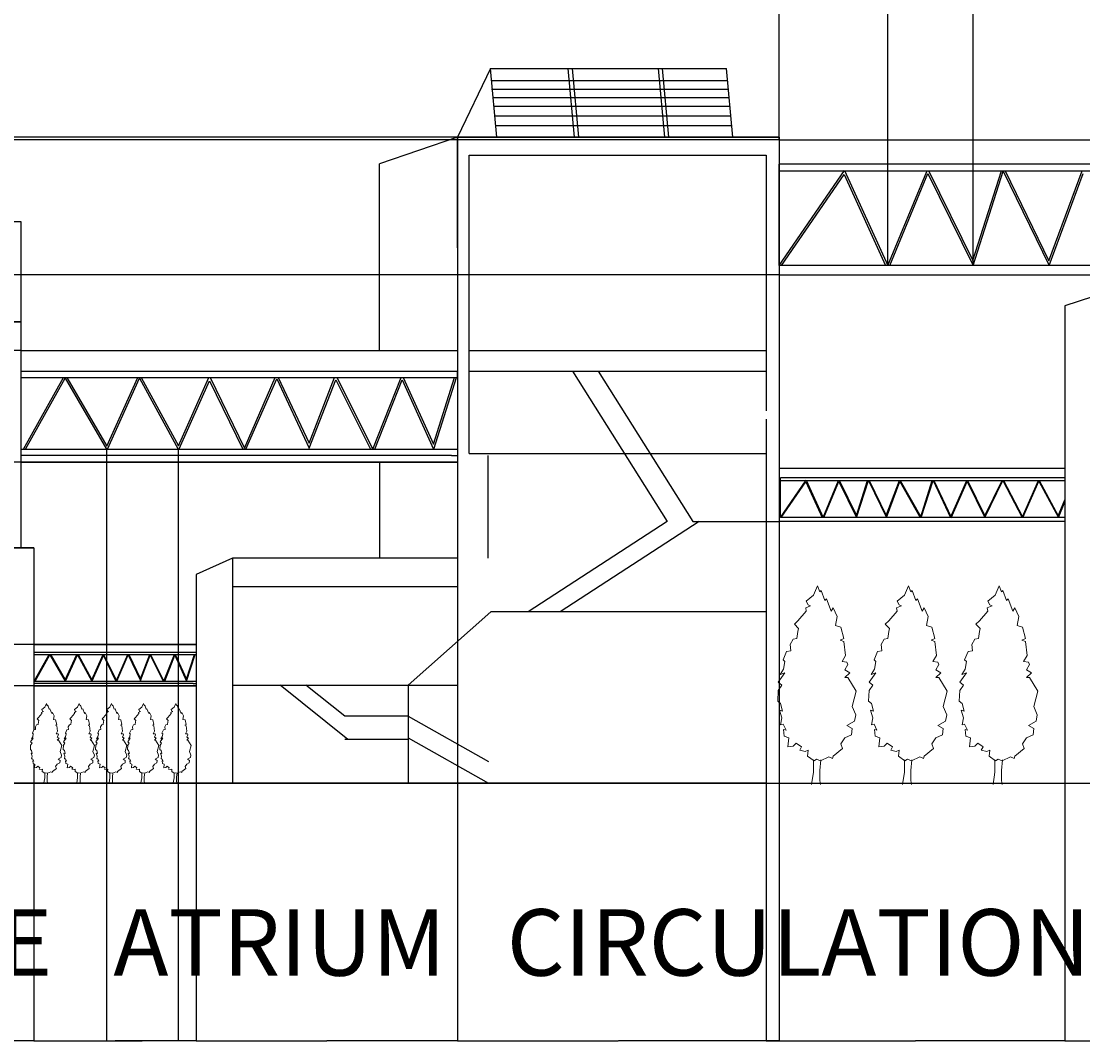
# Model space of a CAD drawing. Units: inches. Extents: x -32109 to 33221, y -19197 to 7608.
# Tile 16 of 25: x 10957 to 19011, y -13530 to -5795. Entities that reach past the tile are written whole.
import ezdxf

# ---------------------------------------------------------------- set-up
doc = ezdxf.new("R2010")
doc.units = ezdxf.units.IN
doc.header["$MEASUREMENT"] = 0
for name, color, linetype, lineweight in [('A-ANNO-DIMS', 2, 'Continuous', 18), ('A-ANNO-TEXT', 7, 'Continuous', 25), ('A-ELEV', 7, 'Continuous', 25), ('L-PLNT', 3, 'Continuous', 13)]:
    doc.layers.add(name, color=color, linetype=linetype, lineweight=lineweight)
doc.styles.get("Standard").update_dxf_attribs({"font": 'arial.ttf'})
doc.dimstyles.get("Standard").update_dxf_attribs({"dimtxt": 0.18, "dimasz": 0.18, "dimexe": 0.18, "dimexo": 0.0625, "dimgap": 0.09, "dimtad": 0, "dimtih": 1, "dimtoh": 1, "dimdec": 4, "dimzin": 0, "dimdsep": 46, "dimtxsty": 'Standard', "dimcen": 0.09, "dimadec": 0, "dimazin": 0, "dimtfac": 1, "dimtdec": 4, "dimtofl": 0, "dimtmove": 0, "dimatfit": 3, "dimfxl": 1, "dimtolj": 1, "dimtzin": 0, "dimarcsym": 0})

# ---------------------------------------------------------------- blocks, each defined once
blk = doc.blocks.new('*U2')
blk.add_lwpolyline([(-2.754, 191.699), (-6.78, 182.851), (-13.682, 176.953), (-11.956, 173.266), (-9.656, 172.529), (-14.257, 170.317), (-13.682, 167.368), (-21.733, 157.783), (-25.184, 154.834), (-21.158, 150.41), (-21.733, 147.461), (-22.884, 140.825), (-26.334, 140.087), (-29.21, 134.926), (-28.635, 129.028), (-32.661, 128.291), (-36.111, 120.18), (-34.386, 118.706), (-35.536, 111.333), (-38.987, 106.171), (-34.386, 107.646), (-40.712, 98.798), (-37.261, 95.849), (-40.712, 90.688), (-41.287, 80.366), (-38.412, 78.154), (-36.686, 70.781), (-39.562, 71.518), (-37.261, 64.145), (-38.412, 57.509), (-36.111, 58.247), (-33.236, 52.348), (-35.536, 53.086), (-34.961, 46.45), (-30.36, 44.975), (-31.51, 36.128), (-26.334, 36.865), (-23.459, 39.814), (-18.283, 36.128), (-20.008, 33.178), (-14.832, 31.704), (-11.956, 33.178), (-12.531, 27.28), (-6.205, 22.856), (-3.905, 24.331), (0.121, 22.856), (8.173, 26.543), (11.624, 25.068), (12.199, 27.28), (21.4, 34.653), (19.675, 39.077), (23.701, 44.975), (30.027, 47.924), (30.602, 53.823), (25.426, 56.772), (32.903, 61.196), (34.053, 67.094), (30.602, 75.205), (34.628, 89.951), (26.576, 103.222), (23.701, 103.222), (28.302, 107.646), (23.701, 110.595), (26.576, 115.756), (25.426, 117.968), (20.825, 118.706), (24.276, 124.604), (22.551, 137.876), (19.1, 139.35), (22.551, 140.825), (19.675, 151.884), (14.499, 153.359), (16.224, 162.207), (12.199, 170.317), (10.473, 167.368), (5.872, 179.165), (4.147, 177.69), (0.696, 187.275), (-0.454, 185.8)], close=True)
for points in [[(-6.813, 23.669), (-6.813, 11.669), (-8.627, 0)], [(0.387, 23.669), (-0.576, 13.271), (-0.576, 3.686), (0, 0)]]:
    blk.add_lwpolyline(points)
blk = doc.blocks.new('*D16')
at = {"layer": 'A-ANNO-DIMS', "color": 0, "lineweight": -2, "transparency": 16777216}
for p, q in [((7931.9, -8929), (7931.9, -4467.1)), ((7932, -4467.3), (18774.7, -4467.3)), ((29618.2, -4467.3), (18775.5, -4467.3)), ((29618.3, -6090.7), (29618.3, -4467.1))]:
    blk.add_line(p, q, dxfattribs=at)
at = {"layer": 'A-ANNO-DIMS', "color": 0, "transparency": 16777216}
for points in [[(7932, -4467.2), (7932, -4467.3), (7931.9, -4467.3)], [(29618.2, -4467.2), (29618.2, -4467.3), (29618.3, -4467.3)]]:
    blk.add_solid(points, dxfattribs=at)
at = {"layer": 'Defpoints', "color": 0, "transparency": 16777216}
for p in [(29618.3, -4467.3), (29618.3, -6090.8), (7931.9, -8929.1)]:
    blk.add_point(p, dxfattribs=at)
at = {"layer": 'A-ANNO-DIMS', "color": 0, "transparency": 16777216, "insert": (18775.1, -4467.3), "char_height": 0.18, "attachment_point": 5}
blk.add_mtext('\\A1;21686', dxfattribs=at)
blk = doc.blocks.new('*D17')
at = {"layer": 'A-ANNO-DIMS', "color": 0, "lineweight": -2, "transparency": 16777216}
for p, q in [((29618.4, -6090.8), (33221.1, -6090.8)), ((33220.9, -6091), (33220.9, -8833.1)), ((33220.9, -11575.6), (33220.9, -8833.5)), ((8978.2, -11575.8), (33221.1, -11575.8))]:
    blk.add_line(p, q, dxfattribs=at)
at = {"layer": 'A-ANNO-DIMS', "color": 0, "transparency": 16777216}
for points in [[(33220.9, -6091), (33221, -6091), (33220.9, -6090.8)], [(33220.9, -11575.6), (33221, -11575.6), (33220.9, -11575.8)]]:
    blk.add_solid(points, dxfattribs=at)
at = {"layer": 'Defpoints', "color": 0, "transparency": 16777216}
for p in [(29618.3, -6090.8), (8978.1, -11575.8), (33220.9, -11575.8)]:
    blk.add_point(p, dxfattribs=at)
at = {"layer": 'A-ANNO-DIMS', "color": 0, "transparency": 16777216, "insert": (33220.9, -8833.3), "char_height": 0.18, "attachment_point": 5}
blk.add_mtext('\\A1;5485', dxfattribs=at)
blk = doc.blocks.new('*D18')
at = {"layer": 'A-ANNO-DIMS', "color": 0, "lineweight": -2, "transparency": 16777216}
for p, q in [((16610.1, -11575.9), (16610.1, -13529.7)), ((18874.4, -11575.9), (18874.4, -13529.7)), ((16610.3, -13529.5), (17741.8, -13529.5)), ((18874.2, -13529.5), (17742.7, -13529.5))]:
    blk.add_line(p, q, dxfattribs=at)
at = {"layer": 'A-ANNO-DIMS', "color": 0, "transparency": 16777216}
for points in [[(16610.3, -13529.5), (16610.3, -13529.5), (16610.1, -13529.5)], [(18874.2, -13529.5), (18874.2, -13529.5), (18874.4, -13529.5)]]:
    blk.add_solid(points, dxfattribs=at)
at = {"layer": 'Defpoints', "color": 0, "transparency": 16777216}
for p in [(16610.1, -11575.8), (18874.4, -11575.8), (18874.4, -13529.5)]:
    blk.add_point(p, dxfattribs=at)
at = {"layer": 'A-ANNO-DIMS', "color": 0, "transparency": 16777216, "insert": (17742.2, -13529.5), "char_height": 0.18, "attachment_point": 5}
blk.add_mtext('\\A1;2264.3', dxfattribs=at)
blk = doc.blocks.new('*D19')
at = {"layer": 'A-ANNO-DIMS', "color": 0, "lineweight": -2, "transparency": 16777216}
for p, q in [((16706.7, -6693.3), (16706.7, -4467.1)), ((16706.9, -4467.3), (21231.6, -4467.3)), ((25757.1, -4467.3), (21232.3, -4467.3)), ((25757.3, -6693.3), (25757.3, -4467.1))]:
    blk.add_line(p, q, dxfattribs=at)
at = {"layer": 'A-ANNO-DIMS', "color": 0, "transparency": 16777216}
for points in [[(16706.9, -4467.2), (16706.9, -4467.3), (16706.7, -4467.3)], [(25757.1, -4467.2), (25757.1, -4467.3), (25757.3, -4467.3)]]:
    blk.add_solid(points, dxfattribs=at)
at = {"layer": 'Defpoints', "color": 0, "transparency": 16777216}
for p in [(25757.3, -4467.3), (16706.7, -6693.4), (25757.3, -6693.4)]:
    blk.add_point(p, dxfattribs=at)
at = {"layer": 'A-ANNO-DIMS', "color": 0, "transparency": 16777216, "insert": (21232, -4467.3), "char_height": 0.18, "attachment_point": 5}
blk.add_mtext('\\A1;9051', dxfattribs=at)
blk = doc.blocks.new('*D119')
at = {"layer": 'A-ANNO-DIMS', "color": 0, "lineweight": -2, "transparency": 16777216}
for p, q in [((8978.1, -11575.9), (8978.1, -13529.7)), ((11053.8, -11575.9), (11053.8, -13529.7)), ((8978.3, -13529.5), (10015.5, -13529.5)), ((11053.6, -13529.5), (10016.4, -13529.5))]:
    blk.add_line(p, q, dxfattribs=at)
at = {"layer": 'A-ANNO-DIMS', "color": 0, "transparency": 16777216}
for points in [[(8978.3, -13529.5), (8978.3, -13529.5), (8978.1, -13529.5)], [(11053.6, -13529.5), (11053.6, -13529.5), (11053.8, -13529.5)]]:
    blk.add_solid(points, dxfattribs=at)
at = {"layer": 'Defpoints', "color": 0, "transparency": 16777216}
for p in [(8978.1, -11575.8), (11053.8, -11575.8), (11053.8, -13529.5)]:
    blk.add_point(p, dxfattribs=at)
at = {"layer": 'A-ANNO-DIMS', "color": 0, "transparency": 16777216, "insert": (10016, -13529.5), "char_height": 0.18, "attachment_point": 5}
blk.add_mtext('\\A1;2075.7', dxfattribs=at)
blk = doc.blocks.new('*D120')
at = {"layer": 'A-ANNO-DIMS', "color": 0, "lineweight": -2, "transparency": 16777216}
for p, q in [((11053.8, -11575.9), (11053.8, -13529.7)), ((12283.6, -11575.9), (12283.6, -13529.7)), ((11054, -13529.5), (11668.2, -13529.5)), ((12283.4, -13529.5), (11669.1, -13529.5))]:
    blk.add_line(p, q, dxfattribs=at)
at = {"layer": 'A-ANNO-DIMS', "color": 0, "transparency": 16777216}
for points in [[(11054, -13529.5), (11054, -13529.5), (11053.8, -13529.5)], [(12283.4, -13529.5), (12283.4, -13529.5), (12283.6, -13529.5)]]:
    blk.add_solid(points, dxfattribs=at)
at = {"layer": 'Defpoints', "color": 0, "transparency": 16777216}
for p in [(11053.8, -11575.8), (12283.6, -11575.8), (12283.6, -13529.5)]:
    blk.add_point(p, dxfattribs=at)
at = {"layer": 'A-ANNO-DIMS', "color": 0, "transparency": 16777216, "insert": (11668.7, -13529.5), "char_height": 0.18, "attachment_point": 5}
blk.add_mtext('\\A1;1229.7', dxfattribs=at)
blk = doc.blocks.new('*D121')
at = {"layer": 'A-ANNO-DIMS', "color": 0, "lineweight": -2, "transparency": 16777216}
for p, q in [((14268.3, -6674.3), (14268.3, -13529.7)), ((12283.6, -11575.9), (12283.6, -13529.7)), ((12283.7, -13529.5), (13275.5, -13529.5)), ((14268.1, -13529.5), (13276.4, -13529.5))]:
    blk.add_line(p, q, dxfattribs=at)
at = {"layer": 'A-ANNO-DIMS', "color": 0, "transparency": 16777216}
for points in [[(12283.7, -13529.5), (12283.7, -13529.5), (12283.6, -13529.5)], [(14268.1, -13529.5), (14268.1, -13529.5), (14268.3, -13529.5)]]:
    blk.add_solid(points, dxfattribs=at)
at = {"layer": 'Defpoints', "color": 0, "transparency": 16777216}
for p in [(14268.3, -6674.3), (12283.6, -11575.8), (14268.3, -13529.5)]:
    blk.add_point(p, dxfattribs=at)
at = {"layer": 'A-ANNO-DIMS', "color": 0, "transparency": 16777216, "insert": (13275.9, -13529.5), "char_height": 0.18, "attachment_point": 5}
blk.add_mtext('\\A1;1984.7', dxfattribs=at)
blk = doc.blocks.new('*D122')
at = {"layer": 'A-ANNO-DIMS', "color": 0, "lineweight": -2, "transparency": 16777216}
for p, q in [((14268.3, -6674.3), (14268.3, -13529.7)), ((16706.7, -6674.3), (16706.7, -13529.7)), ((14268.5, -13529.5), (15487, -13529.5)), ((16706.5, -13529.5), (15488, -13529.5))]:
    blk.add_line(p, q, dxfattribs=at)
at = {"layer": 'A-ANNO-DIMS', "color": 0, "transparency": 16777216}
for points in [[(14268.5, -13529.5), (14268.5, -13529.5), (14268.3, -13529.5)], [(16706.5, -13529.5), (16706.5, -13529.5), (16706.7, -13529.5)]]:
    blk.add_solid(points, dxfattribs=at)
at = {"layer": 'Defpoints', "color": 0, "transparency": 16777216}
for p in [(14268.3, -6674.3), (16706.7, -6674.3), (16706.7, -13529.5)]:
    blk.add_point(p, dxfattribs=at)
at = {"layer": 'A-ANNO-DIMS', "color": 0, "transparency": 16777216, "insert": (15487.5, -13529.5), "char_height": 0.18, "attachment_point": 5}
blk.add_mtext('\\A1;2438.4', dxfattribs=at)
blk = doc.blocks.new('*D124')
at = {"layer": 'A-ANNO-DIMS', "color": 0, "lineweight": -2, "transparency": 16777216}
for p, q in [((10957.6, -7316.5), (5225.4, -7316.5)), ((5225.5, -7316.7), (5225.5, -7696.2)), ((5225.5, -8075.9), (5225.5, -7696.5)), ((10957.6, -8076.1), (5225.4, -8076.1))]:
    blk.add_line(p, q, dxfattribs=at)
at = {"layer": 'A-ANNO-DIMS', "color": 0, "transparency": 16777216}
for points in [[(5225.5, -7316.7), (5225.6, -7316.7), (5225.5, -7316.5)], [(5225.5, -8075.9), (5225.6, -8075.9), (5225.5, -8076.1)]]:
    blk.add_solid(points, dxfattribs=at)
at = {"layer": 'Defpoints', "color": 0, "transparency": 16777216}
for p in [(10957.6, -7316.5), (5225.5, -8076.1), (10957.6, -8076.1)]:
    blk.add_point(p, dxfattribs=at)
at = {"layer": 'A-ANNO-DIMS', "color": 0, "transparency": 16777216, "insert": (5225.5, -7696.3), "char_height": 0.18, "attachment_point": 5}
blk.add_mtext('\\A1;759.6', dxfattribs=at)
blk = doc.blocks.new('*D125')
at = {"layer": 'A-ANNO-DIMS', "color": 0, "lineweight": -2, "transparency": 16777216}
for p, q in [((11053.8, -9789.4), (5225.4, -9789.4)), ((5225.5, -9789.6), (5225.5, -10682.4)), ((5225.5, -11575.6), (5225.5, -10682.8)), ((11053.8, -11575.8), (5225.4, -11575.8))]:
    blk.add_line(p, q, dxfattribs=at)
at = {"layer": 'A-ANNO-DIMS', "color": 0, "transparency": 16777216}
for points in [[(5225.5, -9789.6), (5225.6, -9789.6), (5225.5, -9789.4)], [(5225.5, -11575.6), (5225.6, -11575.6), (5225.5, -11575.8)]]:
    blk.add_solid(points, dxfattribs=at)
at = {"layer": 'Defpoints', "color": 0, "transparency": 16777216}
for p in [(11053.8, -9789.4), (5225.5, -11575.8), (11053.8, -11575.8)]:
    blk.add_point(p, dxfattribs=at)
at = {"layer": 'A-ANNO-DIMS', "color": 0, "transparency": 16777216, "insert": (5225.5, -10682.6), "char_height": 0.18, "attachment_point": 5}
blk.add_mtext('\\A1;1786.4', dxfattribs=at)
blk = doc.blocks.new('*D128')
at = {"layer": 'A-ANNO-DIMS', "color": 0, "lineweight": -2, "transparency": 16777216}
for p, q in [((10957.5, -8293.1), (5225.4, -8293.1)), ((5225.5, -8293.3), (5225.5, -8717)), ((5225.5, -9141), (5225.5, -8717.4)), ((10957.5, -9141.2), (5225.4, -9141.2))]:
    blk.add_line(p, q, dxfattribs=at)
at = {"layer": 'A-ANNO-DIMS', "color": 0, "transparency": 16777216}
for points in [[(5225.5, -8293.3), (5225.6, -8293.3), (5225.5, -8293.1)], [(5225.5, -9141), (5225.6, -9141), (5225.5, -9141.2)]]:
    blk.add_solid(points, dxfattribs=at)
at = {"layer": 'Defpoints', "color": 0, "transparency": 16777216}
for p in [(10957.6, -8293.1), (5225.5, -9141.2), (10957.6, -9141.2)]:
    blk.add_point(p, dxfattribs=at)
at = {"layer": 'A-ANNO-DIMS', "color": 0, "transparency": 16777216, "insert": (5225.5, -8717.2), "char_height": 0.18, "attachment_point": 5}
blk.add_mtext('\\A1;848.1', dxfattribs=at)
blk = doc.blocks.new('*D129')
at = {"layer": 'A-ANNO-DIMS', "color": 0, "lineweight": -2, "transparency": 16777216}
for p, q in [((14268.2, -9141.2), (5225.4, -9141.2)), ((5225.5, -9141.4), (5225.5, -10358.3)), ((5225.5, -11575.6), (5225.5, -10358.7)), ((12283.5, -11575.8), (5225.4, -11575.8))]:
    blk.add_line(p, q, dxfattribs=at)
at = {"layer": 'A-ANNO-DIMS', "color": 0, "transparency": 16777216}
for points in [[(5225.5, -9141.4), (5225.6, -9141.4), (5225.5, -9141.2)], [(5225.5, -11575.6), (5225.6, -11575.6), (5225.5, -11575.8)]]:
    blk.add_solid(points, dxfattribs=at)
at = {"layer": 'Defpoints', "color": 0, "transparency": 16777216}
for p in [(14268.3, -9141.2), (5225.5, -11575.8), (12283.6, -11575.8)]:
    blk.add_point(p, dxfattribs=at)
at = {"layer": 'A-ANNO-DIMS', "color": 0, "transparency": 16777216, "insert": (5225.5, -10358.5), "char_height": 0.18, "attachment_point": 5}
blk.add_mtext('\\A1;2434.6', dxfattribs=at)
blk = doc.blocks.new('*D130')
at = {"layer": 'A-ANNO-DIMS', "color": 0, "lineweight": -2, "transparency": 16777216}
for p, q in [((12283.5, -10522.9), (5225.4, -10522.9)), ((5225.5, -10523.1), (5225.5, -10680.1)), ((5225.5, -10837.4), (5225.5, -10680.4)), ((12283.5, -10837.6), (5225.4, -10837.6))]:
    blk.add_line(p, q, dxfattribs=at)
at = {"layer": 'A-ANNO-DIMS', "color": 0, "transparency": 16777216}
for points in [[(5225.5, -10523.1), (5225.6, -10523.1), (5225.5, -10522.9)], [(5225.5, -10837.4), (5225.6, -10837.4), (5225.5, -10837.6)]]:
    blk.add_solid(points, dxfattribs=at)
at = {"layer": 'Defpoints', "color": 0, "transparency": 16777216}
for p in [(12283.6, -10522.9), (5225.5, -10837.6), (12283.6, -10837.6)]:
    blk.add_point(p, dxfattribs=at)
at = {"layer": 'A-ANNO-DIMS', "color": 0, "transparency": 16777216, "insert": (5225.5, -10680.2), "char_height": 0.18, "attachment_point": 5}
blk.add_mtext('\\A1;314.7', dxfattribs=at)
blk = doc.blocks.new('*D131')
at = {"layer": 'A-ANNO-DIMS', "color": 0, "lineweight": -2, "transparency": 16777216}
for p, q in [((16706.6, -6674.3), (5225.4, -6674.3)), ((5225.5, -6674.4), (5225.5, -9124.9)), ((5225.5, -11575.6), (5225.5, -9125.2)), ((16610, -11575.8), (5225.4, -11575.8))]:
    blk.add_line(p, q, dxfattribs=at)
at = {"layer": 'A-ANNO-DIMS', "color": 0, "transparency": 16777216}
for points in [[(5225.5, -6674.4), (5225.6, -6674.4), (5225.5, -6674.3)], [(5225.5, -11575.6), (5225.6, -11575.6), (5225.5, -11575.8)]]:
    blk.add_solid(points, dxfattribs=at)
at = {"layer": 'Defpoints', "color": 0, "transparency": 16777216}
for p in [(16706.7, -6674.3), (5225.5, -11575.8), (16610.1, -11575.8)]:
    blk.add_point(p, dxfattribs=at)
at = {"layer": 'A-ANNO-DIMS', "color": 0, "transparency": 16777216, "insert": (5225.5, -9125), "char_height": 0.18, "attachment_point": 5}
blk.add_mtext('\\A1;4902', dxfattribs=at)
blk = doc.blocks.new('*D132')
at = {"layer": 'A-ANNO-DIMS', "color": 0, "lineweight": -2, "transparency": 16777216}
for p, q in [((16706.6, -6693.4), (5225.4, -6693.4)), ((5225.5, -6693.6), (5225.5, -7206.4)), ((5225.5, -7719.5), (5225.5, -7206.7)), ((16706.6, -7719.7), (5225.4, -7719.7))]:
    blk.add_line(p, q, dxfattribs=at)
at = {"layer": 'A-ANNO-DIMS', "color": 0, "transparency": 16777216}
for points in [[(5225.5, -6693.6), (5225.6, -6693.6), (5225.5, -6693.4)], [(5225.5, -7719.5), (5225.6, -7719.5), (5225.5, -7719.7)]]:
    blk.add_solid(points, dxfattribs=at)
at = {"layer": 'Defpoints', "color": 0, "transparency": 16777216}
for p in [(16706.7, -6693.4), (5225.5, -7719.7), (16706.7, -7719.7)]:
    blk.add_point(p, dxfattribs=at)
at = {"layer": 'A-ANNO-DIMS', "color": 0, "transparency": 16777216, "insert": (5225.5, -7206.5), "char_height": 0.18, "attachment_point": 5}
blk.add_mtext('\\A1;1026.3', dxfattribs=at)
blk = doc.blocks.new('*D133')
at = {"layer": 'A-ANNO-DIMS', "color": 0, "lineweight": -2, "transparency": 16777216}
for p, q in [((16706.6, -7719.7), (5225.4, -7719.7)), ((5225.5, -7719.9), (5225.5, -9647.6)), ((5225.5, -11575.6), (5225.5, -9647.9)), ((16610, -11575.8), (5225.4, -11575.8))]:
    blk.add_line(p, q, dxfattribs=at)
at = {"layer": 'A-ANNO-DIMS', "color": 0, "transparency": 16777216}
for points in [[(5225.5, -7719.9), (5225.6, -7719.9), (5225.5, -7719.7)], [(5225.5, -11575.6), (5225.6, -11575.6), (5225.5, -11575.8)]]:
    blk.add_solid(points, dxfattribs=at)
at = {"layer": 'Defpoints', "color": 0, "transparency": 16777216}
for p in [(16706.7, -7719.7), (5225.5, -11575.8), (16610.1, -11575.8)]:
    blk.add_point(p, dxfattribs=at)
at = {"layer": 'A-ANNO-DIMS', "color": 0, "transparency": 16777216, "insert": (5225.5, -9647.8), "char_height": 0.18, "attachment_point": 5}
blk.add_mtext('\\A1;3856', dxfattribs=at)
blk = doc.blocks.new('*D134')
at = {"layer": 'A-ANNO-DIMS', "color": 0, "lineweight": -2, "transparency": 16777216}
for p, q in [((11603.4, -9042.1), (11603.4, -13529.7)), ((12147.5, -9042.1), (12147.5, -13529.7)), ((11603.6, -13529.5), (11875.1, -13529.5)), ((12147.3, -13529.5), (11875.8, -13529.5))]:
    blk.add_line(p, q, dxfattribs=at)
at = {"layer": 'A-ANNO-DIMS', "color": 0, "transparency": 16777216}
for points in [[(11603.6, -13529.5), (11603.6, -13529.5), (11603.4, -13529.5)], [(12147.3, -13529.5), (12147.3, -13529.5), (12147.5, -13529.5)]]:
    blk.add_solid(points, dxfattribs=at)
at = {"layer": 'Defpoints', "color": 0, "transparency": 16777216}
for p in [(11603.4, -9042.1), (12147.5, -9042.1), (12147.5, -13529.5)]:
    blk.add_point(p, dxfattribs=at)
at = {"layer": 'A-ANNO-DIMS', "color": 0, "transparency": 16777216, "insert": (11875.5, -13529.5), "char_height": 0.18, "attachment_point": 5}
blk.add_mtext('\\A1;544.1', dxfattribs=at)
blk = doc.blocks.new('*D135')
at = {"layer": 'A-ANNO-DIMS', "color": 0, "lineweight": -2, "transparency": 16777216}
for p, q in [((18874.4, -11575.9), (18874.4, -13529.7)), ((19422.7, -11575.9), (19422.7, -13529.7)), ((18874.5, -13529.5), (19148.2, -13529.5)), ((19422.6, -13529.5), (19148.9, -13529.5))]:
    blk.add_line(p, q, dxfattribs=at)
at = {"layer": 'A-ANNO-DIMS', "color": 0, "transparency": 16777216}
for points in [[(18874.5, -13529.5), (18874.5, -13529.5), (18874.4, -13529.5)], [(19422.6, -13529.5), (19422.6, -13529.5), (19422.7, -13529.5)]]:
    blk.add_solid(points, dxfattribs=at)
at = {"layer": 'Defpoints', "color": 0, "transparency": 16777216}
for p in [(18874.4, -11575.8), (19422.7, -11575.8), (19422.7, -13529.5)]:
    blk.add_point(p, dxfattribs=at)
at = {"layer": 'A-ANNO-DIMS', "color": 0, "transparency": 16777216, "insert": (19148.6, -13529.5), "char_height": 0.18, "attachment_point": 5}
blk.add_mtext('\\A1;548.4', dxfattribs=at)
blk = doc.blocks.new('*D152')
at = {"layer": 'A-ANNO-DIMS', "color": 0, "lineweight": -2, "transparency": 16777216}
for p, q in [((17531.2, -7648.2), (17531.2, -4467.1)), ((17531.3, -4467.3), (17854.5, -4467.3)), ((18178.5, -4467.3), (17855.3, -4467.3)), ((18178.7, -7648.2), (18178.7, -4467.1))]:
    blk.add_line(p, q, dxfattribs=at)
at = {"layer": 'A-ANNO-DIMS', "color": 0, "transparency": 16777216}
for points in [[(17531.3, -4467.2), (17531.3, -4467.3), (17531.2, -4467.3)], [(18178.5, -4467.2), (18178.5, -4467.3), (18178.7, -4467.3)]]:
    blk.add_solid(points, dxfattribs=at)
at = {"layer": 'Defpoints', "color": 0, "transparency": 16777216}
for p in [(18178.7, -4467.3), (17531.2, -7648.3), (18178.7, -7648.3)]:
    blk.add_point(p, dxfattribs=at)
at = {"layer": 'A-ANNO-DIMS', "color": 0, "transparency": 16777216, "insert": (17854.9, -4467.3), "char_height": 0.18, "attachment_point": 5}
blk.add_mtext('\\A1;647.5', dxfattribs=at)

msp = doc.modelspace()

# ---------------------------------------------------------------- linework, layer by layer
at = {"layer": 'A-ELEV'}
for p, q in [((14517.432, -6152.504), (14268.281, -6674.26)), ((14565.284, -6674.26), (14517.432, -6152.504)), ((14517.432, -6152.504), (16307.647, -6152.504)), ((15153.851, -6674.26), (15106, -6152.504)), ((15153.851, -6674.26), (15106, -6152.504)), ((15187.584, -6674.26), (15139.733, -6152.504)), ((15839.437, -6674.26), (15791.585, -6152.504)), ((15871.025, -6674.26), (15823.173, -6152.504)), ((16355.499, -6674.26), (16307.647, -6152.504)), ((14525.941, -6245.283), (16316.156, -6245.283)), ((14525.941, -6309.524), (16322.048, -6309.524)), ((14537.725, -6373.765), (16327.94, -6373.765)), ((14543.617, -6438.006), (16333.831, -6438.006)), ((14550.35, -6511.424), (16340.565, -6511.424)), ((14557.083, -6584.842), (16347.298, -6584.842)), ((14268.281, -6674.26), (13676.029, -6876.602)), ((14268.281, -7512.982), (14268.281, -6674.26)), ((14268.281, -6674.26), (16706.692, -6674.26)), ((16706.692, -6674.26), (16706.692, -9589.972)), ((16706.692, -6693.38), (25757.257, -6693.38)), ((14354.588, -9074.869), (14354.588, -6810.436)), ((14354.588, -6810.436), (16610.1, -6810.436)), ((14354.588, -6810.436), (16610.1, -6810.436)), ((16610.1, -6810.436), (16610.1, -8750.63)), ((13676.029, -8293.138), (13676.029, -6876.602)), ((25757.257, -6878.434), (16706.692, -6878.434)), ((16706.692, -7648.023), (16706.692, -6878.434)), ((16706.692, -7648.023), (17203.3, -6927.833)), ((16706.692, -6930.594), (25757.257, -6930.594)), ((16724.127, -7648.023), (17200.732, -6956.843)), ((17200.732, -6956.843), (17515.281, -7648.023)), ((17203.3, -6927.833), (17531.159, -7648.26)), ((17531.159, -7648.26), (17828.281, -6933.974)), ((17546.804, -7648.023), (17836.694, -6951.122)), ((17836.694, -6951.122), (18178.681, -7648.26)), ((17841.168, -6927.652), (18175.88, -7609.959)), ((18175.88, -7609.959), (18393.537, -6930.594)), ((18178.681, -7648.26), (18408.182, -6931.927)), ((18408.182, -6931.927), (18756.533, -7648.26)), ((18423.495, -6930.594), (18754.741, -7611.755)), ((18754.741, -7611.755), (19006.907, -6930.594)), ((18756.533, -7648.26), (19015.15, -6949.673)), ((10957.64, -7316.541), (9060.882, -7316.541)), ((10957.64, -8076.124), (10957.64, -7316.541)), ((14268.281, -7512.982), (14268.281, -8359.901)), ((25729.008, -7648.023), (16706.692, -7648.023)), ((16706.692, -7719.715), (25729.008, -7719.715)), ((19422.731, -7777.04), (18874.37, -7952.783)), ((18874.37, -7952.783), (18874.37, -9241.759)), ((9060.882, -8076.124), (10957.64, -8076.124)), ((10957.64, -9789.375), (10957.64, -8076.124)), ((10957.576, -8293.138), (14268.281, -8293.138)), ((14354.588, -8292.478), (16610.1, -8292.478)), ((14268.281, -8359.901), (14268.281, -9074.869)), ((10957.576, -8450.266), (14268.281, -8450.266)), ((14268.281, -8497.236), (14268.281, -8450.266)), ((14354.588, -8450.266), (16610.1, -8450.266)), ((14354.588, -8450.266), (16610.1, -8450.266)), ((15139.732, -8450.266), (15857.619, -9589.972)), ((15335.269, -8450.266), (16053.155, -9589.972)), ((10957.576, -8497.236), (14268.281, -8497.236)), ((10973.838, -9042.08), (11277.737, -8497.236)), ((10990.274, -9042.08), (11290.499, -8503.822)), ((11290.499, -8503.822), (11603.428, -9042.08)), ((11303.273, -8497.236), (11606.824, -9019.364)), ((11606.824, -9019.364), (11842.021, -8497.236)), ((11612.663, -9041.351), (11854.744, -8503.941)), ((11854.744, -8503.941), (12147.494, -9042.08)), ((11867.437, -8497.236), (12150.072, -9016.782)), ((12150.072, -9016.782), (12381.591, -8497.236)), ((12155.825, -9039.136), (12386.224, -8522.105)), ((12386.224, -8522.105), (12639, -9042.08)), ((12390.095, -8497.236), (12650.689, -9033.293)), ((12650.689, -9033.293), (12884.714, -8497.236)), ((12662.514, -9042.08), (12895.455, -8508.509)), ((12895.455, -8508.509), (13142.888, -9033.293)), ((12906.009, -8497.236), (13141.601, -8996.907)), ((13141.601, -8996.907), (13335.347, -8497.236)), ((13142.888, -9033.293), (13343.738, -8515.3)), ((13343.738, -8515.3), (13607.68, -9042.08)), ((13350.742, -8497.236), (13623.734, -9042.08)), ((13623.734, -9042.08), (13840.337, -8496.854)), ((13639.179, -9042.08), (13848.534, -8515.096)), ((13848.534, -8515.096), (14085.351, -9042.08)), ((13856.245, -8497.236), (14084.256, -9004.624)), ((14084.256, -9004.624), (14245.281, -8497.236)), ((14087.428, -9042.08), (14260.295, -8497.379)), ((16610.1, -8813.89), (16610.1, -9528.412)), ((16610.184, -8813.89), (16610.1, -8813.89)), ((10957.576, -9042.08), (14221.522, -9042.08)), ((14221.522, -9088.359), (10957.576, -9088.359)), ((14221.522, -9042.08), (14268.281, -9042.08)), ((14221.522, -9088.359), (14268.281, -9088.359)), ((14268.281, -9088.359), (14268.281, -9869.618)), ((14354.588, -9074.869), (16610.1, -9074.869)), ((14497.235, -9088.359), (14497.235, -9869.618)), ((10957.576, -9141.225), (14268.281, -9141.225)), ((13676.029, -9141.225), (13676.029, -9869.618)), ((16706.692, -9185.537), (18874.37, -9185.537)), ((16716.991, -9560.155), (16716.991, -9258.155)), ((18874.37, -9258.155), (16716.991, -9258.155)), ((18874.37, -9241.759), (18874.37, -11575.804)), ((16716.991, -9560.155), (16911.868, -9277.541)), ((16716.991, -9278.624), (18874.37, -9278.624)), ((16723.833, -9560.155), (16910.86, -9288.924)), ((16910.86, -9288.924), (17034.294, -9560.155)), ((16911.868, -9277.541), (17040.525, -9560.248)), ((17040.525, -9560.248), (17157.121, -9279.95)), ((17046.665, -9560.155), (17160.422, -9286.68)), ((17160.422, -9286.68), (17294.624, -9560.248)), ((17162.178, -9277.469), (17293.525, -9545.218)), ((17293.525, -9545.218), (17378.937, -9278.624)), ((17294.624, -9560.248), (17384.684, -9279.147)), ((17384.684, -9279.147), (17521.383, -9560.248)), ((17390.693, -9278.624), (17520.68, -9545.923)), ((17520.68, -9545.923), (17619.634, -9278.624)), ((17521.383, -9560.248), (17622.868, -9286.111)), ((17622.868, -9286.111), (17778.424, -9560.155)), ((17625.425, -9279.205), (17781.65, -9554.428)), ((17781.65, -9554.428), (17868.997, -9278.624)), ((17785.745, -9560.155), (17874.786, -9279)), ((17874.786, -9279), (18008.479, -9560.301)), ((17880.843, -9278.624), (18013.566, -9557.883)), ((18008.479, -9560.301), (18131.594, -9279.038)), ((18013.639, -9562.56), (18134.83, -9285.692)), ((18134.83, -9285.692), (18268.404, -9560.334)), ((18137.656, -9278.624), (18268.391, -9547.428)), ((18268.391, -9547.428), (18398.449, -9278.624)), ((18268.404, -9560.334), (18404.475, -9279.102)), ((18404.475, -9279.102), (18550.106, -9560.364)), ((18410.57, -9278.624), (18553.023, -9553.747)), ((18553.023, -9553.747), (18674.079, -9279.145)), ((18556.353, -9560.155), (18677.47, -9285.417)), ((18677.47, -9285.417), (18826.126, -9560.371)), ((18680.2, -9278.624), (18825.402, -9547.189)), ((18825.402, -9547.189), (18874.37, -9426.661)), ((18826.126, -9560.371), (18874.37, -9441.626)), ((16610.1, -9528.412), (16610.1, -11575.804)), ((18874.37, -9560.155), (16716.991, -9560.155)), ((18550.106, -9560.364), (18550.198, -9560.155)), ((15857.619, -9589.972), (14804.441, -10275.755)), ((16100.087, -9589.972), (15046.91, -10275.755)), ((16053.155, -9589.972), (16706.692, -9589.972)), ((16706.692, -9588.288), (18874.37, -9588.288)), ((8978.112, -9789.375), (11053.825, -9789.375)), ((11053.825, -9789.375), (11053.825, -11170.757)), ((12560.542, -9869.618), (12283.552, -9992.261)), ((14268.281, -9869.618), (12560.542, -9869.618)), ((12560.542, -9869.618), (12560.542, -11575.804)), ((12283.552, -9992.261), (12283.552, -10522.895)), ((14268.281, -10086.432), (12560.542, -10086.432)), ((14519.409, -10275.755), (13894.215, -10831.294)), ((14804.441, -10275.755), (14519.409, -10275.755)), ((16610.1, -10275.755), (14804.441, -10275.755)), ((11053.825, -10522.895), (12283.552, -10522.895)), ((12283.552, -10522.895), (12283.552, -11575.804)), ((11053.825, -10581.198), (12283.552, -10581.198)), ((11053.825, -10598.626), (12283.552, -10598.626)), ((11056.853, -10800.793), (11169.616, -10598.626)), ((11062.952, -10800.793), (11174.351, -10601.07)), ((11174.351, -10601.07), (11290.465, -10800.793)), ((11179.091, -10598.626), (11291.725, -10792.364)), ((11291.725, -10792.364), (11378.996, -10598.626)), ((11293.892, -10800.522), (11383.717, -10601.114)), ((11383.717, -10601.114), (11492.342, -10800.793)), ((11388.426, -10598.626), (11493.299, -10791.406)), ((11493.299, -10791.406), (11579.205, -10598.626)), ((11495.434, -10799.7), (11580.924, -10607.854)), ((11580.924, -10607.854), (11674.718, -10800.793)), ((11582.36, -10598.626), (11679.055, -10797.532)), ((11679.055, -10797.532), (11765.891, -10598.626)), ((11683.443, -10800.793), (11769.876, -10602.809)), ((11769.876, -10602.809), (11861.687, -10797.532)), ((11773.792, -10598.626), (11861.209, -10784.031)), ((11861.209, -10784.031), (11933.1, -10598.626)), ((11861.687, -10797.532), (11936.213, -10605.329)), ((11936.213, -10605.329), (12034.149, -10800.793)), ((11938.812, -10598.626), (12040.107, -10800.793)), ((12040.107, -10800.793), (12120.478, -10598.485)), ((12045.838, -10800.793), (12123.519, -10605.253)), ((12123.519, -10605.253), (12211.391, -10800.793)), ((12126.38, -10598.626), (12210.985, -10786.894)), ((12210.985, -10786.894), (12270.734, -10598.626)), ((12212.162, -10800.793), (12276.305, -10598.68)), ((11053.825, -10800.793), (12261.918, -10800.793)), ((12261.918, -10817.965), (11053.825, -10817.965)), ((11053.825, -10837.581), (12283.552, -10837.581)), ((12212.162, -10800.793), (12279.268, -10800.793)), ((12261.918, -10817.965), (12283.552, -10817.965)), ((12560.542, -10831.294), (14268.281, -10831.294)), ((13434.691, -11243.108), (12920.812, -10831.294)), ((13413.08, -11067.963), (13117.755, -10831.294)), ((13413.08, -11067.963), (13117.755, -10831.294)), ((13894.215, -10831.294), (13894.215, -11575.804)), ((13894.215, -11067.963), (13413.08, -11067.963)), ((13894.215, -11067.963), (14502.226, -11411.619)), ((13894.215, -11243.108), (13413.08, -11243.108)), ((13894.215, -11232.147), (14502.226, -11575.804)), ((11053.825, -11428.689), (11053.825, -11575.804)), ((6605.54, -11575.804), (31840.935, -11575.804)), ((11053.825, -11575.804), (8978.112, -11575.804)), ((11053.825, -11575.804), (20871.064, -11575.804)), ((12560.542, -11575.804), (12733.753, -11575.804)), ((13894.215, -11575.804), (13980.522, -11575.804))]:
    msp.add_line(p, q, dxfattribs=at)

# ---------------------------------------------------------------- block references
at = {"layer": 'L-PLNT'}
for p, xscale, yscale, zscale in [((17020.823, -11584.626), 7.857670648127824, 7.857670648127824, 7.857670648127824), ((17710.925, -11584.626), 7.857670648127824, 7.857670648127824, 7.857670648127824), ((18398.654, -11584.626), 7.857670648127824, 7.857670648127824, 7.857670648127824), ((11156.679, -11572.205), 3.136663191868353, 3.136663191868353, 3.136663191868353), ((11405.326, -11572.205), 3.136663191868353, 3.136663191868353, 3.136663191868353), ((11650.745, -11572.205), 3.136663191868353, 3.136663191868353, 3.136663191868353), ((11892.933, -11572.205), 3.136663191868353, 3.136663191868353, 3.136663191868353), ((12138.352, -11572.205), 3.136663191868353, 3.136663191868353, 3.136663191868353)]:
    msp.add_blockref('*U2', p, dxfattribs=dict(at, xscale=xscale, yscale=yscale, zscale=zscale))

# ---------------------------------------------------------------- texts
at = {"layer": 'A-ANNO-TEXT'}
msp.add_text('SIDE  PROFILE   ATRIUM   CIRCULATION   AND   VERTICAL   CIRCULATION   HUB', height=504.21831, dxfattribs=at).set_placement((6653.092, -13035.812))

# ---------------------------------------------------------------- dimensions: what is measured, and where the dimension line sits
at = {"layer": 'A-ANNO-DIMS'}
for base, p1, p2, override, picture, middle in [((29618.33, -4467.266), (7931.857, -8929.065), (29618.33, -6090.794), {"dimdec": 0, "dimlfac": 1, "dimrnd": 0, "dimzin": 0, "dimdsep": 46, "dimlunit": 2}, '*D16', (18775.094, -4467.266)), ((25757.257, -4467.266), (16706.692, -6693.38), (25757.257, -6693.38), {"dimdec": 0, "dimlfac": 1, "dimrnd": 0, "dimzin": 0, "dimdsep": 46, "dimlunit": 2}, '*D19', (21231.975, -4467.266)), ((18178.681, -4467.266), (17531.159, -7648.26), (18178.681, -7648.26), {"dimdec": 1, "dimlfac": 1, "dimrnd": 0, "dimzin": 0, "dimdsep": 46, "dimlunit": 2}, '*D152', (17854.92, -4467.266)), ((14268.281, -13529.49), (12283.552, -11575.804), (14268.281, -6674.26), {"dimdec": 1, "dimlfac": 1, "dimrnd": 0, "dimzin": 0, "dimdsep": 46, "dimlunit": 2}, '*D121', (13275.916, -13529.49)), ((16706.692, -13529.49), (14268.281, -6674.26), (16706.692, -6674.26), {"dimdec": 1, "dimlfac": 1, "dimrnd": 0, "dimzin": 0, "dimdsep": 46, "dimlunit": 2}, '*D122', (15487.486, -13529.49)), ((12147.494, -13529.49), (11603.428, -9042.08), (12147.494, -9042.08), {"dimdec": 1, "dimlfac": 1, "dimrnd": 0, "dimzin": 0, "dimdsep": 46, "dimlunit": 2}, '*D134', (11875.461, -13529.49)), ((11053.825, -13529.49), (8978.112, -11575.804), (11053.825, -11575.804), {"dimdec": 1, "dimlfac": 1, "dimrnd": 0, "dimzin": 0, "dimdsep": 46, "dimlunit": 2}, '*D119', (10015.969, -13529.49)), ((12283.552, -13529.49), (11053.825, -11575.804), (12283.552, -11575.804), {"dimdec": 1, "dimlfac": 1, "dimrnd": 0, "dimzin": 0, "dimdsep": 46, "dimlunit": 2}, '*D120', (11668.688, -13529.49)), ((18874.37, -13529.49), (16610.1, -11575.804), (18874.37, -11575.804), {"dimdec": 1, "dimlfac": 1, "dimrnd": 0, "dimzin": 0, "dimdsep": 46, "dimlunit": 2}, '*D18', (17742.235, -13529.49)), ((19422.731, -13529.49), (18874.37, -11575.804), (19422.731, -11575.804), {"dimdec": 1, "dimlfac": 1, "dimrnd": 0, "dimzin": 0, "dimdsep": 46, "dimlunit": 2}, '*D135', (19148.55, -13529.49))]:
    dim = msp.add_linear_dim(base=base, p1=p1, p2=p2, dimstyle='Standard', override=override, dxfattribs=at)
    dim.commit()
    dim.dimension.update_dxf_attribs({"geometry": picture, "text_midpoint": middle})
for base, p1, p2, override, picture, middle in [((33220.935, -11575.804), (29618.33, -6090.794), (8978.112, -11575.804), {"dimdec": 0, "dimlfac": 1, "dimrnd": 0, "dimzin": 0, "dimdsep": 46, "dimlunit": 2}, '*D17', (33220.935, -8833.299)), ((5225.54, -11575.804), (16706.692, -6674.26), (16610.1, -11575.804), {"dimdec": 0, "dimlfac": 1, "dimrnd": 0, "dimzin": 0, "dimdsep": 46, "dimlunit": 2}, '*D131', (5225.54, -9125.032)), ((5225.54, -7719.715), (16706.692, -6693.38), (16706.692, -7719.715), {"dimdec": 1, "dimlfac": 1, "dimrnd": 0, "dimzin": 0, "dimdsep": 46, "dimlunit": 2}, '*D132', (5225.54, -7206.547)), ((5225.54, -8076.124), (10957.64, -7316.541), (10957.64, -8076.124), {"dimdec": 1, "dimlfac": 1, "dimrnd": 0, "dimzin": 0, "dimdsep": 46, "dimlunit": 2}, '*D124', (5225.54, -7696.333)), ((5225.54, -11575.804), (16706.692, -7719.715), (16610.1, -11575.804), {"dimdec": 0, "dimlfac": 1, "dimrnd": 0, "dimzin": 0, "dimdsep": 46, "dimlunit": 2}, '*D133', (5225.54, -9647.759)), ((5225.54, -9141.225), (10957.576, -8293.138), (10957.576, -9141.225), {"dimdec": 1, "dimlfac": 1, "dimrnd": 0, "dimzin": 0, "dimdsep": 46, "dimlunit": 2}, '*D128', (5225.54, -8717.181)), ((5225.54, -11575.804), (14268.281, -9141.225), (12283.552, -11575.804), {"dimdec": 1, "dimlfac": 1, "dimrnd": 0, "dimzin": 0, "dimdsep": 46, "dimlunit": 2}, '*D129', (5225.54, -10358.514)), ((5225.54, -11575.804), (11053.825, -9789.375), (11053.825, -11575.804), {"dimdec": 1, "dimlfac": 1, "dimrnd": 0, "dimzin": 0, "dimdsep": 46, "dimlunit": 2}, '*D125', (5225.54, -10682.589)), ((5225.54, -10837.581), (12283.552, -10522.895), (12283.552, -10837.581), {"dimdec": 1, "dimlfac": 1, "dimrnd": 0, "dimzin": 0, "dimdsep": 46, "dimlunit": 2}, '*D130', (5225.54, -10680.238))]:
    dim = msp.add_linear_dim(base=base, p1=p1, p2=p2, angle=90, dimstyle='Standard', override=override, dxfattribs=at)
    dim.commit()
    dim.dimension.update_dxf_attribs({"geometry": picture, "text_midpoint": middle})

doc.saveas('drawing.dxf')
